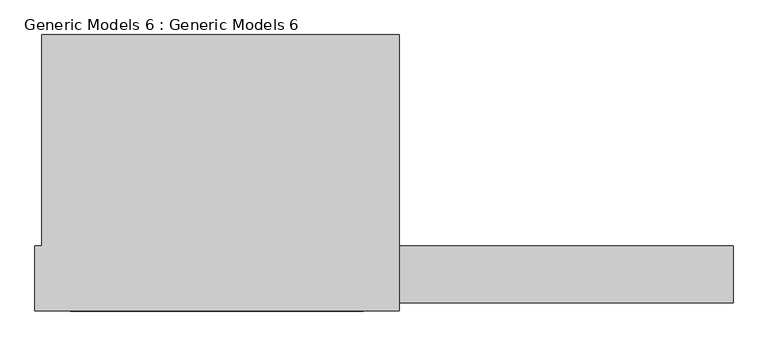
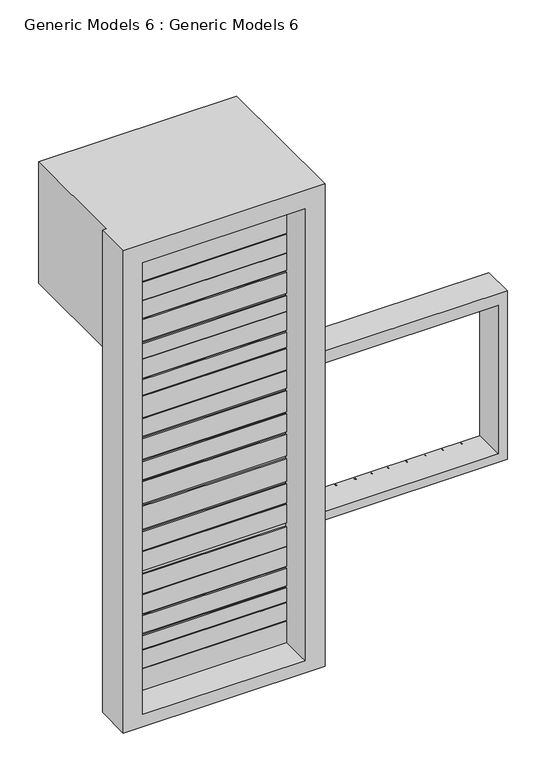
"""IFC4 building model written with IfcOpenShell, lengths in millimetres: proxy geometry, Generic Models 6 : Generic Models 6."""

from ifc_helpers import new_model, si_unit, origin, place, context, project, spatial, faceted_brep, source, transform, mapped, element, save


def generic_models_6_generic_models_6_5a8cbb59(model_context):
    return source(origin(), model_context, "Body", "Brep", [
        faceted_brep([(-14524.7437117, -10819.8592534, 5313.3697962), (-11550.5831929, -10819.8592534, 5313.3697962), (-11550.5831929, -10819.8592534, 2659.3923672), (-14524.7437117, -10819.8592534, 2659.3923672), (-14524.7437117, -10819.8592534, 2506.9923672), (-11398.1831929, -10819.8592534, 2506.9923672), (-11398.1831929, -10819.8592534, 5522.6005165), (-14524.7437117, -10819.8592534, 5522.6005165), (-11398.1831929, -10286.4592534, 5522.6005165), (-14524.7437117, -10286.4592534, 5522.6005165), (-11550.5831929, -10286.4592534, 5313.3697962), (-11550.5831929, -10286.4592534, 2659.3923672), (-11398.1831929, -10286.4592534, 2506.9923672), (-14524.7437117, -10286.4592534, 5313.3697962), (-14524.7437117, -10286.4592534, 2659.3923672), (-14293.7831929, -10311.8592534, 2659.3923672), (-14277.8960614, -10311.8592534, 2659.3923672), (-14277.8960614, -10337.2592534, 2659.3923672), (-14293.7831929, -10337.2592534, 2659.3923672), (-14019.6359859, -10311.8592534, 2659.3923672), (-14004.4843067, -10311.8592534, 2659.3923672), (-14004.4843067, -10337.2592534, 2659.3923672), (-14019.6359859, -10337.2592534, 2659.3923672), (-13695.1641924, -10311.8592534, 2659.3923672), (-13674.725498, -10311.8592534, 2659.3923672), (-13674.725498, -10337.2592534, 2659.3923672), (-13695.1641924, -10337.2592534, 2659.3923672), (-13411.1331929, -10311.8592534, 2659.3923672), (-13398.4331929, -10311.8592534, 2659.3923672), (-13398.4331929, -10337.2592534, 2659.3923672), (-13411.1331929, -10337.2592534, 2659.3923672), (-13132.6036786, -10311.8592534, 2659.3923672), (-13122.8488627, -10311.8592534, 2659.3923672), (-13122.8488627, -10337.2592534, 2659.3923672), (-13132.6036786, -10337.2592534, 2659.3923672), (-12816.2756326, -10311.8592534, 2659.3923672), (-12805.7258669, -10311.8592534, 2659.3923672), (-12805.7258669, -10337.2592534, 2659.3923672), (-12816.2756326, -10337.2592534, 2659.3923672), (-12496.7331929, -10311.8592534, 2659.3923672), (-12491.0846074, -10311.8592534, 2659.3923672), (-12491.0846074, -10337.2592534, 2659.3923672), (-12496.7331929, -10337.2592534, 2659.3923672), (-12209.2160936, -10311.8592534, 2659.3923672), (-12202.6421379, -10311.8592534, 2659.3923672), (-12202.6421379, -10337.2592534, 2659.3923672), (-12209.2160936, -10337.2592534, 2659.3923672), (-11888.3927856, -10311.8592534, 2659.3923672), (-11880.9442119, -10311.8592534, 2659.3923672), (-11880.9442119, -10337.2592534, 2659.3923672), (-11888.3927856, -10337.2592534, 2659.3923672), (-14524.7437117, -10286.4592534, 2506.9923672), (-14277.8960614, -10311.8592534, 2506.9923672), (-14293.7831929, -10311.8592534, 2506.9923672), (-14293.7831929, -10337.2592534, 2506.9923672), (-14277.8960614, -10337.2592534, 2506.9923672), (-14004.4843067, -10311.8592534, 2506.9923672), (-14019.6359859, -10311.8592534, 2506.9923672), (-14019.6359859, -10337.2592534, 2506.9923672), (-14004.4843067, -10337.2592534, 2506.9923672), (-13674.725498, -10311.8592534, 2506.9923672), (-13695.1641924, -10311.8592534, 2506.9923672), (-13695.1641924, -10337.2592534, 2506.9923672), (-13674.725498, -10337.2592534, 2506.9923672), (-13398.4331929, -10311.8592534, 2506.9923672), (-13411.1331929, -10311.8592534, 2506.9923672), (-13411.1331929, -10337.2592534, 2506.9923672), (-13398.4331929, -10337.2592534, 2506.9923672), (-13122.8488627, -10311.8592534, 2506.9923672), (-13132.6036786, -10311.8592534, 2506.9923672), (-13132.6036786, -10337.2592534, 2506.9923672), (-13122.8488627, -10337.2592534, 2506.9923672), (-12805.7258669, -10311.8592534, 2506.9923672), (-12816.2756326, -10311.8592534, 2506.9923672), (-12816.2756326, -10337.2592534, 2506.9923672), (-12805.7258669, -10337.2592534, 2506.9923672), (-12491.0846074, -10311.8592534, 2506.9923672), (-12496.7331929, -10311.8592534, 2506.9923672), (-12496.7331929, -10337.2592534, 2506.9923672), (-12491.0846074, -10337.2592534, 2506.9923672), (-12202.6421379, -10311.8592534, 2506.9923672), (-12209.2160936, -10311.8592534, 2506.9923672), (-12209.2160936, -10337.2592534, 2506.9923672), (-12202.6421379, -10337.2592534, 2506.9923672), (-11880.9442119, -10311.8592534, 2506.9923672), (-11888.3927856, -10311.8592534, 2506.9923672), (-11888.3927856, -10337.2592534, 2506.9923672), (-11880.9442119, -10337.2592534, 2506.9923672), (-14524.7437117, -10896.0592534, 8571.3431053), (-17940.6112417, -10896.0592534, 8571.3431053), (-17940.6112417, -10896.0592534, -50.8), (-14524.7437117, -10896.0592534, -50.8), (-14865.1651398, -10896.0592534, 8244.6595507), (-14865.1651398, -10896.0592534, 167.4595507), (-17608.3651398, -10896.0592534, 167.4595507), (-17608.3651398, -10896.0592534, 8244.6595507), (-14524.7437117, -10286.4592534, -50.8), (-17940.6112417, -10286.4592534, -50.8), (-17940.6112417, -10286.4592534, 8571.3431053), (-17877.5437117, -10286.4592534, 8571.3431053), (-17877.5437117, -10286.4592534, 6400.8), (-14524.7437117, -10286.4592534, 6400.8), (-14524.7437117, -8305.2592534, 8571.3431053), (-17877.5437117, -8305.2592534, 8571.3431053), (-14524.7437117, -8305.2592534, 6400.8), (-14865.1651398, -10362.6592534, 8244.6595507), (-17608.3651398, -10362.6592534, 8244.6595507), (-17608.3651398, -10362.6592534, 7869.8316641), (-14865.1651398, -10362.6592534, 7869.8316641), (-17608.3651398, -10362.6592534, 167.4595507), (-14865.1651398, -10362.6592534, 167.4595507), (-14865.1651398, -10362.6592534, 548.6341726), (-17608.3651398, -10362.6592534, 548.6341726), (-17608.3651398, -10362.6592534, 7851.6706555), (-17608.3651398, -10362.6592534, 7484.3986193), (-14865.1651398, -10362.6592534, 7484.3986193), (-14865.1651398, -10362.6592534, 7851.6706555), (-17608.3651398, -10362.6592534, 7466.652836), (-17608.3651398, -10362.6592534, 7141.3259469), (-14865.1651398, -10362.6592534, 7141.3259469), (-14865.1651398, -10362.6592534, 7466.652836), (-17608.3651398, -10362.6592534, 7130.7333947), (-17608.3651398, -10362.6592534, 6820.8960364), (-14865.1651398, -10362.6592534, 6820.8960364), (-14865.1651398, -10362.6592534, 7130.7333947), (-17608.3651398, -10362.6592534, 6792.059761), (-17608.3651398, -10362.6592534, 6410.2172809), (-14865.1651398, -10362.6592534, 6410.2172809), (-14865.1651398, -10362.6592534, 6792.059761), (-17608.3651398, -10362.6592534, 6367.8001566), (-17608.3651398, -10362.6592534, 6096.0), (-14865.1651398, -10362.6592534, 6096.0), (-14865.1651398, -10362.6592534, 6367.8001566), (-17608.3651398, -10362.6592534, 6083.1954916), (-17608.3651398, -10362.6592534, 5750.8422485), (-14865.1651398, -10362.6592534, 5750.8422485), (-14865.1651398, -10362.6592534, 6083.1954916), (-17608.3651398, -10362.6592534, 5719.3740642), (-17608.3651398, -10362.6592534, 5444.8375202), (-14865.1651398, -10362.6592534, 5444.8375202), (-14865.1651398, -10362.6592534, 5719.3740642), (-17608.3651398, -10362.6592534, 5420.6168384), (-17608.3651398, -10362.6592534, 5044.1737185), (-14865.1651398, -10362.6592534, 5044.1737185), (-14865.1651398, -10362.6592534, 5420.6168384), (-17608.3651398, -10362.6592534, 5024.0574676), (-17608.3651398, -10362.6592534, 4711.7327534), (-14865.1651398, -10362.6592534, 4711.7327534), (-14865.1651398, -10362.6592534, 5024.0574676), (-17608.3651398, -10362.6592534, 4668.6402942), (-17608.3651398, -10362.6592534, 4297.3929422), (-14865.1651398, -10362.6592534, 4297.3929422), (-14865.1651398, -10362.6592534, 4668.6402942), (-17608.3651398, -10362.6592534, 4257.0119133), (-17608.3651398, -10362.6592534, 3934.6390795), (-14865.1651398, -10362.6592534, 3934.6390795), (-14865.1651398, -10362.6592534, 4257.0119133), (-17608.3651398, -10362.6592534, 3894.206255), (-17608.3651398, -10362.6592534, 3507.0931812), (-14865.1651398, -10362.6592534, 3507.0931812), (-14865.1651398, -10362.6592534, 3894.206255), (-17608.3651398, -10362.6592534, 3458.1113218), (-17608.3651398, -10362.6592534, 3048.0), (-14865.1651398, -10362.6592534, 3048.0), (-14865.1651398, -10362.6592534, 3458.1113218), (-17608.3651398, -10362.6592534, 3005.8203398), (-17608.3651398, -10362.6592534, 2664.3672629), (-14865.1651398, -10362.6592534, 2664.3672629), (-14865.1651398, -10362.6592534, 3005.8203398), (-17608.3651398, -10362.6592534, 2640.7532912), (-17608.3651398, -10362.6592534, 2308.4950454), (-14865.1651398, -10362.6592534, 2308.4950454), (-14865.1651398, -10362.6592534, 2640.7532912), (-17608.3651398, -10362.6592534, 2240.1715077), (-17608.3651398, -10362.6592534, 1894.1870147), (-14865.1651398, -10362.6592534, 1894.1870147), (-14865.1651398, -10362.6592534, 2240.1715077), (-17608.3651398, -10362.6592534, 1877.7198068), (-17608.3651398, -10362.6592534, 1535.0658402), (-14865.1651398, -10362.6592534, 1535.0658402), (-14865.1651398, -10362.6592534, 1877.7198068), (-17608.3651398, -10362.6592534, 1500.8288416), (-17608.3651398, -10362.6592534, 1184.7914294), (-14865.1651398, -10362.6592534, 1184.7914294), (-14865.1651398, -10362.6592534, 1500.8288416), (-17608.3651398, -10362.6592534, 1146.4474358), (-17608.3651398, -10362.6592534, 898.7089016), (-14865.1651398, -10362.6592534, 898.7089016), (-14865.1651398, -10362.6592534, 1146.4474358), (-17608.3651398, -10362.6592534, 880.4045738), (-17608.3651398, -10362.6592534, 563.061774), (-14865.1651398, -10362.6592534, 563.061774), (-14865.1651398, -10362.6592534, 880.4045738), (-14865.1651398, -10337.2592534, 7869.8316641), (-14865.1651398, -10337.2592534, 7851.6706555), (-14865.1651398, -10337.2592534, 7484.3986193), (-14865.1651398, -10337.2592534, 7466.652836), (-14865.1651398, -10337.2592534, 7141.3259469), (-14865.1651398, -10337.2592534, 7130.7333947), (-14865.1651398, -10337.2592534, 6820.8960364), (-14865.1651398, -10337.2592534, 6792.059761), (-14865.1651398, -10337.2592534, 6410.2172809), (-14865.1651398, -10337.2592534, 6367.8001566), (-14865.1651398, -10337.2592534, 6096.0), (-14865.1651398, -10337.2592534, 6083.1954916), (-14865.1651398, -10337.2592534, 5750.8422485), (-14865.1651398, -10337.2592534, 5719.3740642), (-14865.1651398, -10337.2592534, 5444.8375202), (-14865.1651398, -10337.2592534, 5420.6168384), (-14865.1651398, -10337.2592534, 5044.1737185), (-14865.1651398, -10337.2592534, 5024.0574676), (-14865.1651398, -10337.2592534, 4711.7327534), (-14865.1651398, -10337.2592534, 4668.6402942), (-14865.1651398, -10337.2592534, 4297.3929422), (-14865.1651398, -10337.2592534, 4257.0119133), (-14865.1651398, -10337.2592534, 3934.6390795), (-14865.1651398, -10337.2592534, 3894.206255), (-14865.1651398, -10337.2592534, 3507.0931812), (-14865.1651398, -10337.2592534, 3458.1113218), (-14865.1651398, -10337.2592534, 3048.0), (-14865.1651398, -10337.2592534, 3005.8203398), (-14865.1651398, -10337.2592534, 2664.3672629), (-14865.1651398, -10337.2592534, 2640.7532912), (-14865.1651398, -10337.2592534, 2308.4950454), (-14865.1651398, -10337.2592534, 2240.1715077), (-14865.1651398, -10337.2592534, 1894.1870147), (-14865.1651398, -10337.2592534, 1877.7198068), (-14865.1651398, -10337.2592534, 1535.0658402), (-14865.1651398, -10337.2592534, 1500.8288416), (-14865.1651398, -10337.2592534, 1184.7914294), (-14865.1651398, -10337.2592534, 1146.4474358), (-14865.1651398, -10337.2592534, 898.7089016), (-14865.1651398, -10337.2592534, 880.4045738), (-14865.1651398, -10337.2592534, 563.061774), (-14865.1651398, -10337.2592534, 548.6341726), (-17608.3651398, -10337.2592534, 548.6341726), (-17608.3651398, -10337.2592534, 563.061774), (-17608.3651398, -10337.2592534, 880.4045738), (-17608.3651398, -10337.2592534, 898.7089016), (-17608.3651398, -10337.2592534, 1146.4474358), (-17608.3651398, -10337.2592534, 1184.7914294), (-17608.3651398, -10337.2592534, 1500.8288416), (-17608.3651398, -10337.2592534, 1535.0658402), (-17608.3651398, -10337.2592534, 1877.7198068), (-17608.3651398, -10337.2592534, 1894.1870147), (-17608.3651398, -10337.2592534, 2240.1715077), (-17608.3651398, -10337.2592534, 2308.4950454), (-17608.3651398, -10337.2592534, 2640.7532912), (-17608.3651398, -10337.2592534, 2664.3672629), (-17608.3651398, -10337.2592534, 3005.8203398), (-17608.3651398, -10337.2592534, 3048.0), (-17608.3651398, -10337.2592534, 3458.1113218), (-17608.3651398, -10337.2592534, 3507.0931812), (-17608.3651398, -10337.2592534, 3894.206255), (-17608.3651398, -10337.2592534, 3934.6390795), (-17608.3651398, -10337.2592534, 4257.0119133), (-17608.3651398, -10337.2592534, 4297.3929422), (-17608.3651398, -10337.2592534, 4668.6402942), (-17608.3651398, -10337.2592534, 4711.7327534), (-17608.3651398, -10337.2592534, 5024.0574676), (-17608.3651398, -10337.2592534, 5044.1737185), (-17608.3651398, -10337.2592534, 5420.6168384), (-17608.3651398, -10337.2592534, 5444.8375202), (-17608.3651398, -10337.2592534, 5719.3740642), (-17608.3651398, -10337.2592534, 5750.8422485), (-17608.3651398, -10337.2592534, 6083.1954916), (-17608.3651398, -10337.2592534, 6096.0), (-17608.3651398, -10337.2592534, 6367.8001566), (-17608.3651398, -10337.2592534, 6410.2172809), (-17608.3651398, -10337.2592534, 6792.059761), (-17608.3651398, -10337.2592534, 6820.8960364), (-17608.3651398, -10337.2592534, 7130.7333947), (-17608.3651398, -10337.2592534, 7141.3259469), (-17608.3651398, -10337.2592534, 7466.652836), (-17608.3651398, -10337.2592534, 7484.3986193), (-17608.3651398, -10337.2592534, 7851.6706555), (-17608.3651398, -10337.2592534, 7869.8316641), (-17877.5437117, -8305.2592534, 6400.8)], [[[0, 1, 2, 3, 4, 5, 6, 7]], [[6, 8, 9, 7]], [[1, 10, 11, 2]], [[8, 6, 5, 12]], [[1, 0, 13, 10]], [[11, 14, 3, 2], [15, 16, 17, 18], [19, 20, 21, 22], [23, 24, 25, 26], [27, 28, 29, 30], [31, 32, 33, 34], [35, 36, 37, 38], [39, 40, 41, 42], [43, 44, 45, 46], [47, 48, 49, 50]], [[5, 4, 51, 12], [52, 53, 54, 55], [56, 57, 58, 59], [60, 61, 62, 63], [64, 65, 66, 67], [68, 69, 70, 71], [72, 73, 74, 75], [76, 77, 78, 79], [80, 81, 82, 83], [84, 85, 86, 87]], [[88, 89, 90, 91], [92, 93, 94, 95]], [[96, 97, 98, 99, 100, 101, 9, 8, 12, 51], [10, 13, 14, 11]], [[89, 88, 102, 103, 99, 98]], [[90, 89, 98, 97]], [[91, 90, 97, 96]], [[88, 91, 96, 51, 4, 3, 14, 13, 0, 7, 9, 101, 104, 102]], [[105, 106, 107, 108]], [[109, 110, 111, 112]], [[113, 114, 115, 116]], [[117, 118, 119, 120]], [[121, 122, 123, 124]], [[125, 126, 127, 128]], [[129, 130, 131, 132]], [[133, 134, 135, 136]], [[137, 138, 139, 140]], [[141, 142, 143, 144]], [[145, 146, 147, 148]], [[149, 150, 151, 152]], [[153, 154, 155, 156]], [[157, 158, 159, 160]], [[161, 162, 163, 164]], [[165, 166, 167, 168]], [[169, 170, 171, 172]], [[173, 174, 175, 176]], [[177, 178, 179, 180]], [[181, 182, 183, 184]], [[185, 186, 187, 188]], [[189, 190, 191, 192]], [[110, 93, 92, 105, 108, 193, 194, 116, 115, 195, 196, 120, 119, 197, 198, 124, 123, 199, 200, 128, 127, 201, 202, 132, 131, 203, 204, 136, 135, 205, 206, 140, 139, 207, 208, 144, 143, 209, 210, 148, 147, 211, 212, 152, 151, 213, 214, 156, 155, 215, 216, 160, 159, 217, 218, 164, 163, 219, 220, 168, 167, 221, 222, 172, 171, 223, 224, 176, 175, 225, 226, 180, 179, 227, 228, 184, 183, 229, 230, 188, 187, 231, 232, 192, 191, 233, 234, 111]], [[110, 109, 94, 93]], [[94, 109, 112, 235, 236, 190, 189, 237, 238, 186, 185, 239, 240, 182, 181, 241, 242, 178, 177, 243, 244, 174, 173, 245, 246, 170, 169, 247, 248, 166, 165, 249, 250, 162, 161, 251, 252, 158, 157, 253, 254, 154, 153, 255, 256, 150, 149, 257, 258, 146, 145, 259, 260, 142, 141, 261, 262, 138, 137, 263, 264, 134, 133, 265, 266, 130, 129, 267, 268, 126, 125, 269, 270, 122, 121, 271, 272, 118, 117, 273, 274, 114, 113, 275, 276, 107, 106, 95]], [[106, 105, 92, 95]], [[100, 277, 104, 101]], [[103, 102, 104, 277]], [[99, 103, 277, 100]], [[15, 53, 52, 16]], [[19, 57, 56, 20]], [[23, 61, 60, 24]], [[27, 65, 64, 28]], [[31, 69, 68, 32]], [[35, 73, 72, 36]], [[39, 77, 76, 40]], [[43, 81, 80, 44]], [[47, 85, 84, 48]], [[17, 55, 54, 18]], [[21, 59, 58, 22]], [[25, 63, 62, 26]], [[29, 67, 66, 30]], [[33, 71, 70, 34]], [[37, 75, 74, 38]], [[41, 79, 78, 42]], [[45, 83, 82, 46]], [[49, 87, 86, 50]], [[16, 52, 55, 17]], [[53, 15, 18, 54]], [[20, 56, 59, 21]], [[57, 19, 22, 58]], [[24, 60, 63, 25]], [[61, 23, 26, 62]], [[28, 64, 67, 29]], [[65, 27, 30, 66]], [[32, 68, 71, 33]], [[69, 31, 34, 70]], [[36, 72, 75, 37]], [[73, 35, 38, 74]], [[40, 76, 79, 41]], [[77, 39, 42, 78]], [[44, 80, 83, 45]], [[81, 43, 46, 82]], [[48, 84, 87, 49]], [[85, 47, 50, 86]], [[193, 276, 275, 194]], [[195, 274, 273, 196]], [[197, 272, 271, 198]], [[199, 270, 269, 200]], [[201, 268, 267, 202]], [[203, 266, 265, 204]], [[205, 264, 263, 206]], [[207, 262, 261, 208]], [[209, 260, 259, 210]], [[211, 258, 257, 212]], [[213, 256, 255, 214]], [[215, 254, 253, 216]], [[217, 252, 251, 218]], [[219, 250, 249, 220]], [[221, 248, 247, 222]], [[223, 246, 245, 224]], [[225, 244, 243, 226]], [[227, 242, 241, 228]], [[229, 240, 239, 230]], [[231, 238, 237, 232]], [[233, 236, 235, 234]], [[194, 275, 113, 116]], [[276, 193, 108, 107]], [[196, 273, 117, 120]], [[274, 195, 115, 114]], [[198, 271, 121, 124]], [[272, 197, 119, 118]], [[200, 269, 125, 128]], [[270, 199, 123, 122]], [[202, 267, 129, 132]], [[268, 201, 127, 126]], [[204, 265, 133, 136]], [[266, 203, 131, 130]], [[206, 263, 137, 140]], [[264, 205, 135, 134]], [[208, 261, 141, 144]], [[262, 207, 139, 138]], [[210, 259, 145, 148]], [[260, 209, 143, 142]], [[212, 257, 149, 152]], [[258, 211, 147, 146]], [[214, 255, 153, 156]], [[256, 213, 151, 150]], [[216, 253, 157, 160]], [[254, 215, 155, 154]], [[218, 251, 161, 164]], [[252, 217, 159, 158]], [[220, 249, 165, 168]], [[250, 219, 163, 162]], [[222, 247, 169, 172]], [[248, 221, 167, 166]], [[224, 245, 173, 176]], [[246, 223, 171, 170]], [[226, 243, 177, 180]], [[244, 225, 175, 174]], [[228, 241, 181, 184]], [[242, 227, 179, 178]], [[230, 239, 185, 188]], [[240, 229, 183, 182]], [[232, 237, 189, 192]], [[238, 231, 187, 186]], [[234, 235, 112, 111]], [[236, 233, 191, 190]]]),
    ])


if __name__ == "__main__":
    model = new_model("IFC4")
    model_context = context("Model", 3, world=origin())
    ifc_project = project(units=[si_unit("LENGTHUNIT", "METRE", prefix="MILLI")], contexts=[model_context])
    site = spatial("IfcSite", under=ifc_project)
    building = spatial("IfcBuilding", under=site)
    placement = place(None, origin())
    generic_models_6_generic_models_6_shape = generic_models_6_generic_models_6_5a8cbb59(model_context)
    element("IfcBuildingElementProxy", 1, Name="Generic Models 6 : Generic Models 6", ObjectType="Generic Models 6 : Generic Models 6", at=placement, inside=building, context=model_context, shape_type="MappedRepresentation", body=[
        mapped(generic_models_6_generic_models_6_shape, transform((0.0, 0.0, 0.0), x_axis=(1.0, 0.0, 0.0), y_axis=(0.0, 1.0, 0.0), z_axis=(0.0, 0.0, 1.0))),
    ])
    save(model, "model.ifc")
